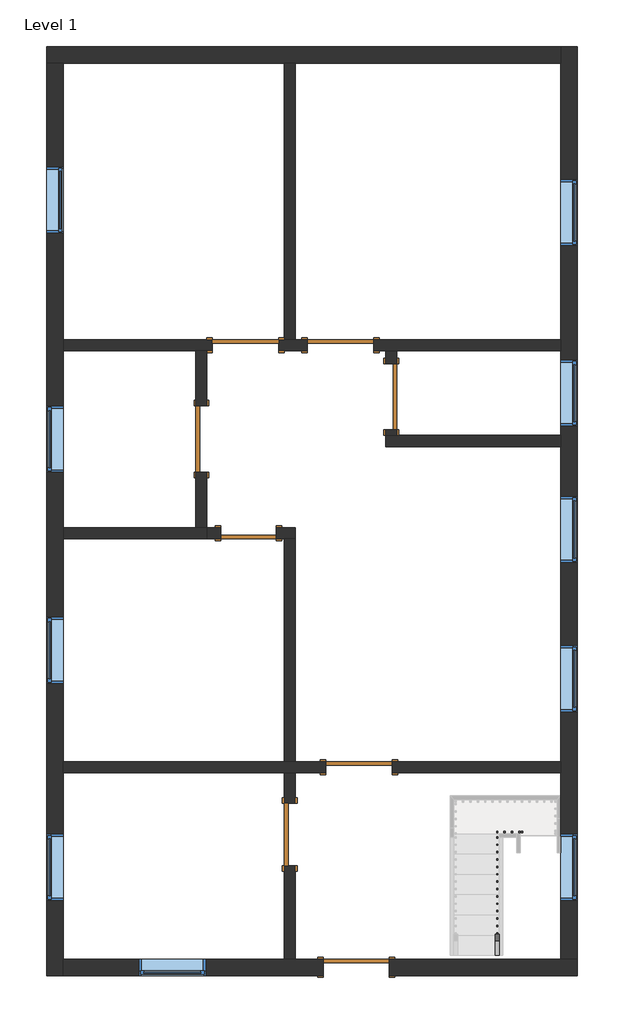
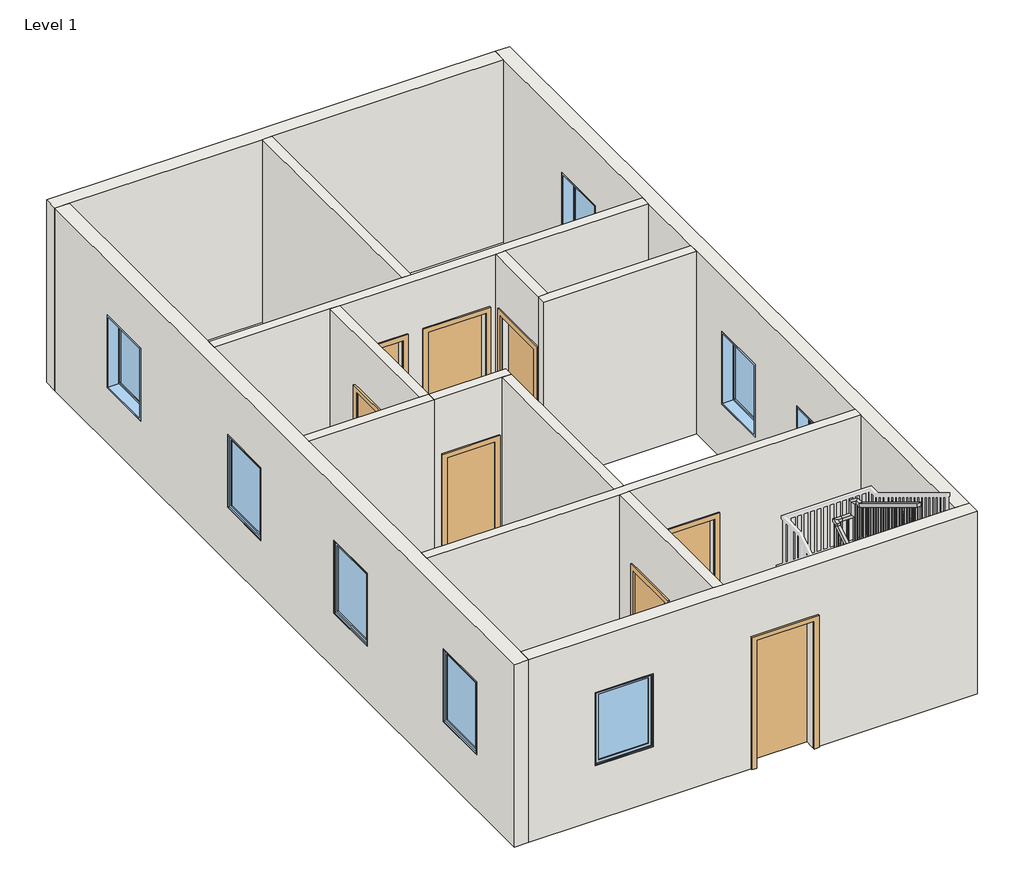
# One storey, part 1 of 2: 13 walls, 10 windows, 8 doors, 1 railing.
"""IFC4 building model written with IfcOpenShell, lengths in millimetres."""

from ifc_helpers import new_model, si_unit, frame, origin, origin_with_axes, place, context, project, spatial, polyline, outline, extrude, faceted_brep, transform, mapped, element, save
from components import door_255cab33, door_56e8e0a9, door_a90ba1ad, door_686f89d2, door_16372e1c, window_c1f32544

model = new_model("IFC4")

# Units and contexts
model_context = context("Model", 3, world=origin())
ifc_project = project(units=[si_unit("LENGTHUNIT", "METRE", prefix="MILLI")], contexts=[model_context])

# Site, building, storey
site = spatial("IfcSite", under=ifc_project)
building = spatial("IfcBuilding", under=site)
storey = spatial("IfcBuildingStorey", under=building, Name="Level 1", Elevation=0.0)

# Doors
placement = place(None, origin())
door_shape = door_255cab33(model_context)
element("IfcDoor", 1, ObjectType="Single-Flush : 30\" x 80\"", at=placement, inside=storey, context=model_context, shape_type="MappedRepresentation", body=[
    mapped(door_shape, transform((-4366.7629117, 1337.2575851, 0.0), x_axis=(1.0, 0.0, 0.0), y_axis=(0.0, 1.0, 0.0), z_axis=(0.0, 0.0, 1.0))),
])
door_2_shape = door_56e8e0a9(model_context)
element("IfcDoor", 2, ObjectType="Single-Flush : 34\" x 80\"", at=placement, inside=storey, context=model_context, shape_type="MappedRepresentation", body=[
    mapped(door_2_shape, transform((-3795.2629117, -2815.6424149, 0.0), x_axis=(0.0, 1.0, 0.0), y_axis=(-1.0, 0.0, 0.0), z_axis=(0.0, 0.0, 1.0))),
])
door_3_shape = door_a90ba1ad(model_context)
element("IfcDoor", 3, ObjectType="Single-Flush : 36\" x 84\"", at=placement, inside=storey, context=model_context, shape_type="MappedRepresentation", body=[
    mapped(door_3_shape, transform((-2880.8629117, -4644.4424149, 0.0), x_axis=(-1.0, 0.0, 0.0), y_axis=(0.0, -1.0, 0.0), z_axis=(0.0, 0.0, 1.0))),
])
door_4_shape = door_686f89d2(model_context)
element("IfcDoor", 4, ObjectType="Single-Flush : 36\" x 84\"", at=placement, inside=storey, context=model_context, shape_type="MappedRepresentation", body=[
    mapped(door_4_shape, transform((-2842.7629117, -1888.5424149, 0.0), x_axis=(-1.0, 0.0, 0.0), y_axis=(0.0, -1.0, 0.0), z_axis=(0.0, 0.0, 1.0))),
])
element("IfcDoor", 5, ObjectType="Single-Flush : 36\" x 84\"", at=placement, inside=storey, context=model_context, shape_type="MappedRepresentation", body=[
    mapped(door_4_shape, transform((-3096.7629117, 3928.0575851, 0.0), x_axis=(-1.0, 0.0, 0.0), y_axis=(0.0, -1.0, 0.0), z_axis=(0.0, 0.0, 1.0))),
])
element("IfcDoor", 6, ObjectType="Single-Flush : 36\" x 84\"", at=placement, inside=storey, context=model_context, shape_type="MappedRepresentation", body=[
    mapped(door_4_shape, transform((-2398.2629117, 3216.8575851, 0.0), x_axis=(0.0, 1.0, 0.0), y_axis=(-1.0, 0.0, 0.0), z_axis=(0.0, 0.0, 1.0))),
])
element("IfcDoor", 7, ObjectType="Single-Flush : 36\" x 84\"", at=placement, inside=storey, context=model_context, shape_type="MappedRepresentation", body=[
    mapped(door_4_shape, transform((-5014.4629117, 2632.6575851, 0.0), x_axis=(0.0, -1.0, 0.0), y_axis=(1.0, 0.0, 0.0), z_axis=(0.0, 0.0, 1.0))),
])
door_5_shape = door_16372e1c(model_context)
element("IfcDoor", 8, ObjectType="Single-Flush : 36\" x 84\"", at=placement, inside=storey, context=model_context, shape_type="MappedRepresentation", body=[
    mapped(door_5_shape, transform((-4404.8629117, 3928.0575851, 0.0), x_axis=(1.0, 0.0, 0.0), y_axis=(0.0, 1.0, 0.0), z_axis=(0.0, 0.0, 1.0))),
])

# Railing
element("IfcRailing", 9, ObjectType="Handrail - Rectangular", at=placement, inside=storey, context=model_context, shape_type="SolidModel", body=[
    faceted_brep([(-963.1629117, -4479.3424149, 1083.7333333), (-963.1629117, -4479.3424149, 1024.3318731), (-912.3629117, -4479.3424149, 1024.3318731), (-912.3629117, -4479.3424149, 1083.7333333), (-963.1629117, -2879.1424149, 2053.5515152), (-963.1629117, -2828.3424149, 2024.9379337), (-912.3629117, -2828.3424149, 2024.9379337), (-912.3629117, -2879.1424149, 2053.5515152), (-963.1629117, -2879.1424149, 2099.7333333), (-963.1629117, -2828.3424149, 2048.9333333), (-912.3629117, -2828.3424149, 2048.9333333), (-912.3629117, -2879.1424149, 2099.7333333), (-963.1629117, -2752.1424149, 2099.7333333), (-963.1629117, -2752.1424149, 2048.9333333), (-912.3629117, -2802.9424149, 2048.9333333), (-912.3629117, -2802.9424149, 2099.7333333), (-836.1629117, -2752.1424149, 2099.7333333), (-836.1629117, -2752.1424149, 2048.9333333), (-836.1629117, -2802.9424149, 2048.9333333), (-836.1629117, -2802.9424149, 2099.7333333), (-696.4629117, -2752.1424149, 2099.7333333), (-645.6629117, -2752.1424149, 2048.9333333), (-645.6629117, -2802.9424149, 2048.9333333), (-696.4629117, -2802.9424149, 2099.7333333), (-696.4629117, -2752.1424149, 2315.2484848), (-645.6629117, -2752.1424149, 2264.4484848), (-645.6629117, -2802.9424149, 2264.4484848), (-696.4629117, -2802.9424149, 2315.2484848), (-569.4629117, -2752.1424149, 2315.2484848), (-569.4629117, -2752.1424149, 2264.4484848), (-620.2629117, -2802.9424149, 2264.4484848), (-620.2629117, -2802.9424149, 2315.2484848), (-569.4629117, -2879.1424149, 2315.2484848), (-569.4629117, -2893.3348244, 2264.4484848), (-620.2629117, -2893.3348244, 2264.4484848), (-620.2629117, -2879.1424149, 2315.2484848), (-569.4629117, -4479.3424149, 3285.0666667), (-620.2629117, -4479.3424149, 3285.0666667), (-620.2629117, -4479.3424149, 3225.6652064), (-569.4629117, -4479.3424149, 3225.6652064)], [[[0, 1, 2, 3]], [[1, 0, 4, 5]], [[2, 1, 5, 6]], [[3, 2, 6, 7]], [[0, 3, 7, 4]], [[5, 4, 8, 9]], [[6, 5, 9, 10]], [[7, 6, 10, 11]], [[4, 7, 11, 8]], [[9, 8, 12, 13]], [[10, 9, 13, 14]], [[11, 10, 14, 15]], [[8, 11, 15, 12]], [[13, 12, 16, 17]], [[14, 13, 17, 18]], [[15, 14, 18, 19]], [[12, 15, 19, 16]], [[17, 16, 20, 21]], [[18, 17, 21, 22]], [[19, 18, 22, 23]], [[16, 19, 23, 20]], [[21, 20, 24, 25]], [[22, 21, 25, 26]], [[23, 22, 26, 27]], [[20, 23, 27, 24]], [[25, 24, 28, 29]], [[26, 25, 29, 30]], [[27, 26, 30, 31]], [[24, 27, 31, 28]], [[29, 28, 32, 33]], [[30, 29, 33, 34]], [[31, 30, 34, 35]], [[28, 31, 35, 32]], [[36, 37, 38, 39]], [[33, 32, 36, 39]], [[34, 33, 39, 38]], [[35, 34, 38, 37]], [[32, 35, 37, 36]]]),
    extrude(outline(polyline([(-4412.6674149, 3185.2561155), (-4393.6174149, 3173.710661), (-4393.6174149, 2201.3333333), (-4412.6674149, 2201.3333333), (-4412.6674149, 3185.2561155)])), frame((-604.3879117, 0.0, 0.0), z_axis=(1.0, 0.0, 0.0), x_axis=(0.0, 1.0, 0.0)), (0.0, 0.0, 1.0), 19.05),
    extrude(outline(polyline([(-4311.0674149, 3123.6803579), (-4292.0174149, 3112.1349034), (-4292.0174149, 2201.3333333), (-4311.0674149, 2201.3333333), (-4311.0674149, 3123.6803579)])), frame((-604.3879117, 0.0, 0.0), z_axis=(1.0, 0.0, 0.0), x_axis=(0.0, 1.0, 0.0)), (0.0, 0.0, 1.0), 19.05),
    extrude(outline(polyline([(-4209.4674149, 3062.1046004), (-4190.4174149, 3050.5591458), (-4190.4174149, 2201.3333333), (-4209.4674149, 2201.3333333), (-4209.4674149, 3062.1046004)])), frame((-604.3879117, 0.0, 0.0), z_axis=(1.0, 0.0, 0.0), x_axis=(0.0, 1.0, 0.0)), (0.0, 0.0, 1.0), 19.05),
    extrude(outline(polyline([(-4107.8674149, 3000.5288428), (-4088.8174149, 2988.9833882), (-4088.8174149, 2032.0), (-4107.8674149, 2032.0), (-4107.8674149, 3000.5288428)])), frame((-604.3879117, 0.0, 0.0), z_axis=(1.0, 0.0, 0.0), x_axis=(0.0, 1.0, 0.0)), (0.0, 0.0, 1.0), 19.05),
    extrude(outline(polyline([(-4006.2674149, 2938.9530852), (-3987.2174149, 2927.4076307), (-3987.2174149, 2032.0), (-4006.2674149, 2032.0), (-4006.2674149, 2938.9530852)])), frame((-604.3879117, 0.0, 0.0), z_axis=(1.0, 0.0, 0.0), x_axis=(0.0, 1.0, 0.0)), (0.0, 0.0, 1.0), 19.05),
    extrude(outline(polyline([(-3904.6674149, 2877.3773276), (-3885.6174149, 2865.8318731), (-3885.6174149, 1862.6666667), (-3904.6674149, 1862.6666667), (-3904.6674149, 2877.3773276)])), frame((-604.3879117, 0.0, 0.0), z_axis=(1.0, 0.0, 0.0), x_axis=(0.0, 1.0, 0.0)), (0.0, 0.0, 1.0), 19.05),
    extrude(outline(polyline([(-3803.0674149, 2815.80157), (-3784.0174149, 2804.2561155), (-3784.0174149, 1862.6666667), (-3803.0674149, 1862.6666667), (-3803.0674149, 2815.80157)])), frame((-604.3879117, 0.0, 0.0), z_axis=(1.0, 0.0, 0.0), x_axis=(0.0, 1.0, 0.0)), (0.0, 0.0, 1.0), 19.05),
    extrude(outline(polyline([(-3701.4674149, 2754.2258125), (-3682.4174149, 2742.6803579), (-3682.4174149, 1862.6666667), (-3701.4674149, 1862.6666667), (-3701.4674149, 2754.2258125)])), frame((-604.3879117, 0.0, 0.0), z_axis=(1.0, 0.0, 0.0), x_axis=(0.0, 1.0, 0.0)), (0.0, 0.0, 1.0), 19.05),
    extrude(outline(polyline([(-3599.8674149, 2692.6500549), (-3580.8174149, 2681.1046004), (-3580.8174149, 1693.3333333), (-3599.8674149, 1693.3333333), (-3599.8674149, 2692.6500549)])), frame((-604.3879117, 0.0, 0.0), z_axis=(1.0, 0.0, 0.0), x_axis=(0.0, 1.0, 0.0)), (0.0, 0.0, 1.0), 19.05),
    extrude(outline(polyline([(-3498.2674149, 2631.0742973), (-3479.2174149, 2619.5288428), (-3479.2174149, 1693.3333333), (-3498.2674149, 1693.3333333), (-3498.2674149, 2631.0742973)])), frame((-604.3879117, 0.0, 0.0), z_axis=(1.0, 0.0, 0.0), x_axis=(0.0, 1.0, 0.0)), (0.0, 0.0, 1.0), 19.05),
    extrude(outline(polyline([(-3396.6674149, 2569.4985397), (-3377.6174149, 2557.9530852), (-3377.6174149, 1693.3333333), (-3396.6674149, 1693.3333333), (-3396.6674149, 2569.4985397)])), frame((-604.3879117, 0.0, 0.0), z_axis=(1.0, 0.0, 0.0), x_axis=(0.0, 1.0, 0.0)), (0.0, 0.0, 1.0), 19.05),
    extrude(outline(polyline([(-3295.0674149, 2507.9227822), (-3276.0174149, 2496.3773276), (-3276.0174149, 1524.0), (-3295.0674149, 1524.0), (-3295.0674149, 2507.9227822)])), frame((-604.3879117, 0.0, 0.0), z_axis=(1.0, 0.0, 0.0), x_axis=(0.0, 1.0, 0.0)), (0.0, 0.0, 1.0), 19.05),
    extrude(outline(polyline([(-3193.4674149, 2446.3470246), (-3174.4174149, 2434.80157), (-3174.4174149, 1524.0), (-3193.4674149, 1524.0), (-3193.4674149, 2446.3470246)])), frame((-604.3879117, 0.0, 0.0), z_axis=(1.0, 0.0, 0.0), x_axis=(0.0, 1.0, 0.0)), (0.0, 0.0, 1.0), 19.05),
    extrude(outline(polyline([(-3091.8674149, 2384.771267), (-3072.8174149, 2373.2258125), (-3072.8174149, 1524.0), (-3091.8674149, 1524.0), (-3091.8674149, 2384.771267)])), frame((-604.3879117, 0.0, 0.0), z_axis=(1.0, 0.0, 0.0), x_axis=(0.0, 1.0, 0.0)), (0.0, 0.0, 1.0), 19.05),
    extrude(outline(polyline([(-2990.2674149, 2323.1955094), (-2971.2174149, 2311.6500549), (-2971.2174149, 1354.6666667), (-2990.2674149, 1354.6666667), (-2990.2674149, 2323.1955094)])), frame((-604.3879117, 0.0, 0.0), z_axis=(1.0, 0.0, 0.0), x_axis=(0.0, 1.0, 0.0)), (0.0, 0.0, 1.0), 19.05),
    extrude(outline(polyline([(-2888.6674149, 2261.6197519), (-2869.6174149, 2250.0742973), (-2869.6174149, 1354.6666667), (-2888.6674149, 1354.6666667), (-2888.6674149, 2261.6197519)])), frame((-604.3879117, 0.0, 0.0), z_axis=(1.0, 0.0, 0.0), x_axis=(0.0, 1.0, 0.0)), (0.0, 0.0, 1.0), 19.05),
    extrude(outline(polyline([(-642.4879117, -2787.0674149), (-642.4879117, -2768.0174149), (-623.4379117, -2768.0174149), (-623.4379117, -2787.0674149), (-642.4879117, -2787.0674149)])), frame((0.0, 0.0, 1185.3333333), z_axis=(0.0, 0.0, 1.0), x_axis=(1.0, 0.0, 0.0)), (0.0, 0.0, 1.0), 1079.1151515),
    extrude(outline(polyline([(-744.0879117, -2787.0674149), (-744.0879117, -2768.0174149), (-725.0379117, -2768.0174149), (-725.0379117, -2787.0674149), (-744.0879117, -2787.0674149)])), frame((0.0, 0.0, 1185.3333333), z_axis=(0.0, 0.0, 1.0), x_axis=(1.0, 0.0, 0.0)), (0.0, 0.0, 1.0), 863.6),
    extrude(outline(polyline([(-845.6879117, -2787.0674149), (-845.6879117, -2768.0174149), (-826.6379117, -2768.0174149), (-826.6379117, -2787.0674149), (-845.6879117, -2787.0674149)])), frame((0.0, 0.0, 1185.3333333), z_axis=(0.0, 0.0, 1.0), x_axis=(1.0, 0.0, 0.0)), (0.0, 0.0, 1.0), 863.6),
    extrude(outline(polyline([(-928.2379117, -2863.2674149), (-947.2879117, -2863.2674149), (-947.2879117, -2844.2174149), (-928.2379117, -2844.2174149), (-928.2379117, -2863.2674149)])), frame((0.0, 0.0, 1016.0), z_axis=(0.0, 0.0, 1.0), x_axis=(1.0, 0.0, 0.0)), (0.0, 0.0, 1.0), 1032.9333333),
    extrude(outline(polyline([(-2964.8674149, 1942.1955094), (-2945.8174149, 1953.740964), (-2945.8174149, 1016.0), (-2964.8674149, 1016.0), (-2964.8674149, 1942.1955094)])), frame((-947.2879117, 0.0, 0.0), z_axis=(1.0, 0.0, 0.0), x_axis=(0.0, 1.0, 0.0)), (0.0, 0.0, 1.0), 19.05),
    extrude(outline(polyline([(-3066.4674149, 1880.6197519), (-3047.4174149, 1892.1652064), (-3047.4174149, 1016.0), (-3066.4674149, 1016.0), (-3066.4674149, 1880.6197519)])), frame((-947.2879117, 0.0, 0.0), z_axis=(1.0, 0.0, 0.0), x_axis=(0.0, 1.0, 0.0)), (0.0, 0.0, 1.0), 19.05),
    extrude(outline(polyline([(-3168.0674149, 1819.0439943), (-3149.0174149, 1830.5894488), (-3149.0174149, 846.6666667), (-3168.0674149, 846.6666667), (-3168.0674149, 1819.0439943)])), frame((-947.2879117, 0.0, 0.0), z_axis=(1.0, 0.0, 0.0), x_axis=(0.0, 1.0, 0.0)), (0.0, 0.0, 1.0), 19.05),
    extrude(outline(polyline([(-3269.6674149, 1757.4682367), (-3250.6174149, 1769.0136913), (-3250.6174149, 846.6666667), (-3269.6674149, 846.6666667), (-3269.6674149, 1757.4682367)])), frame((-947.2879117, 0.0, 0.0), z_axis=(1.0, 0.0, 0.0), x_axis=(0.0, 1.0, 0.0)), (0.0, 0.0, 1.0), 19.05),
    extrude(outline(polyline([(-3371.2674149, 1695.8924791), (-3352.2174149, 1707.4379337), (-3352.2174149, 846.6666667), (-3371.2674149, 846.6666667), (-3371.2674149, 1695.8924791)])), frame((-947.2879117, 0.0, 0.0), z_axis=(1.0, 0.0, 0.0), x_axis=(0.0, 1.0, 0.0)), (0.0, 0.0, 1.0), 19.05),
    extrude(outline(polyline([(-3472.8674149, 1634.3167216), (-3453.8174149, 1645.8621761), (-3453.8174149, 677.3333333), (-3472.8674149, 677.3333333), (-3472.8674149, 1634.3167216)])), frame((-947.2879117, 0.0, 0.0), z_axis=(1.0, 0.0, 0.0), x_axis=(0.0, 1.0, 0.0)), (0.0, 0.0, 1.0), 19.05),
    extrude(outline(polyline([(-3574.4674149, 1572.740964), (-3555.4174149, 1584.2864185), (-3555.4174149, 677.3333333), (-3574.4674149, 677.3333333), (-3574.4674149, 1572.740964)])), frame((-947.2879117, 0.0, 0.0), z_axis=(1.0, 0.0, 0.0), x_axis=(0.0, 1.0, 0.0)), (0.0, 0.0, 1.0), 19.05),
    extrude(outline(polyline([(-3676.0674149, 1511.1652064), (-3657.0174149, 1522.710661), (-3657.0174149, 508.0), (-3676.0674149, 508.0), (-3676.0674149, 1511.1652064)])), frame((-947.2879117, 0.0, 0.0), z_axis=(1.0, 0.0, 0.0), x_axis=(0.0, 1.0, 0.0)), (0.0, 0.0, 1.0), 19.05),
    extrude(outline(polyline([(-3777.6674149, 1449.5894488), (-3758.6174149, 1461.1349034), (-3758.6174149, 508.0), (-3777.6674149, 508.0), (-3777.6674149, 1449.5894488)])), frame((-947.2879117, 0.0, 0.0), z_axis=(1.0, 0.0, 0.0), x_axis=(0.0, 1.0, 0.0)), (0.0, 0.0, 1.0), 19.05),
    extrude(outline(polyline([(-3879.2674149, 1388.0136913), (-3860.2174149, 1399.5591458), (-3860.2174149, 508.0), (-3879.2674149, 508.0), (-3879.2674149, 1388.0136913)])), frame((-947.2879117, 0.0, 0.0), z_axis=(1.0, 0.0, 0.0), x_axis=(0.0, 1.0, 0.0)), (0.0, 0.0, 1.0), 19.05),
    extrude(outline(polyline([(-3980.8674149, 1326.4379337), (-3961.8174149, 1337.9833882), (-3961.8174149, 338.6666667), (-3980.8674149, 338.6666667), (-3980.8674149, 1326.4379337)])), frame((-947.2879117, 0.0, 0.0), z_axis=(1.0, 0.0, 0.0), x_axis=(0.0, 1.0, 0.0)), (0.0, 0.0, 1.0), 19.05),
    extrude(outline(polyline([(-4082.4674149, 1264.8621761), (-4063.4174149, 1276.4076307), (-4063.4174149, 338.6666667), (-4082.4674149, 338.6666667), (-4082.4674149, 1264.8621761)])), frame((-947.2879117, 0.0, 0.0), z_axis=(1.0, 0.0, 0.0), x_axis=(0.0, 1.0, 0.0)), (0.0, 0.0, 1.0), 19.05),
    extrude(outline(polyline([(-4184.0674149, 1203.2864185), (-4165.0174149, 1214.8318731), (-4165.0174149, 338.6666667), (-4184.0674149, 338.6666667), (-4184.0674149, 1203.2864185)])), frame((-947.2879117, 0.0, 0.0), z_axis=(1.0, 0.0, 0.0), x_axis=(0.0, 1.0, 0.0)), (0.0, 0.0, 1.0), 19.05),
    extrude(outline(polyline([(-4285.6674149, 1141.710661), (-4266.6174149, 1153.2561155), (-4266.6174149, 169.3333333), (-4285.6674149, 169.3333333), (-4285.6674149, 1141.710661)])), frame((-947.2879117, 0.0, 0.0), z_axis=(1.0, 0.0, 0.0), x_axis=(0.0, 1.0, 0.0)), (0.0, 0.0, 1.0), 19.05),
    extrude(outline(polyline([(-4387.2674149, 1080.1349034), (-4368.2174149, 1091.6803579), (-4368.2174149, 169.3333333), (-4387.2674149, 169.3333333), (-4387.2674149, 1080.1349034)])), frame((-947.2879117, 0.0, 0.0), z_axis=(1.0, 0.0, 0.0), x_axis=(0.0, 1.0, 0.0)), (0.0, 0.0, 1.0), 19.05),
    extrude(outline(polyline([(-604.3879117, -2787.0674149), (-604.3879117, -2768.0174149), (-585.3379117, -2768.0174149), (-585.3379117, -2787.0674149), (-604.3879117, -2787.0674149)])), frame((0.0, 0.0, 1185.3333333), z_axis=(0.0, 0.0, 1.0), x_axis=(1.0, 0.0, 0.0)), (0.0, 0.0, 1.0), 1079.1151515),
    extrude(outline(polyline([(-928.2379117, -2787.0674149), (-947.2879117, -2787.0674149), (-947.2879117, -2768.0174149), (-928.2379117, -2768.0174149), (-928.2379117, -2787.0674149)])), frame((0.0, 0.0, 1185.3333333), z_axis=(0.0, 0.0, 1.0), x_axis=(1.0, 0.0, 0.0)), (0.0, 0.0, 1.0), 863.6),
    extrude(outline(polyline([(-4479.3424149, 3225.6652064), (-4460.2924149, 3214.1197519), (-4460.2924149, 2201.3333333), (-4479.3424149, 2201.3333333), (-4479.3424149, 3225.6652064)])), frame((-604.3879117, 0.0, 0.0), z_axis=(1.0, 0.0, 0.0), x_axis=(0.0, 1.0, 0.0)), (0.0, 0.0, 1.0), 19.05),
    extrude(outline(polyline([(-4479.3424149, 1024.3318731), (-4460.2924149, 1035.8773276), (-4460.2924149, 169.3333333), (-4479.3424149, 169.3333333), (-4479.3424149, 1024.3318731)])), frame((-947.2879117, 0.0, 0.0), z_axis=(1.0, 0.0, 0.0), x_axis=(0.0, 1.0, 0.0)), (0.0, 0.0, 1.0), 19.05),
])

# Walls
element("IfcWall", 10, ObjectType="Generic - 6\"", at=placement, inside=storey, context=model_context, shape_type="SweptSolid", body=[
    extrude(outline(polyline([(-3719.0629117, 7814.2575851), (-3719.0629117, 4004.2575851), (-3871.4629117, 4004.2575851), (-3871.4629117, 7814.2575851), (-3719.0629117, 7814.2575851)])), origin_with_axes(), (0.0, 0.0, 1.0), 3048.0),
])
element("IfcWall", 11, ObjectType="Generic - 6\"", at=placement, inside=storey, context=model_context, shape_type="Brep", body=[
    faceted_brep([(-3947.6629117, 3851.8575851, 2133.6), (-3947.6629117, 3851.8575851, 0.0), (-3553.9629117, 3851.8575851, 0.0), (-3553.9629117, 3851.8575851, 2133.6), (-2639.5629117, 3851.8575851, 2133.6), (-2639.5629117, 3851.8575851, 0.0), (-2474.4629117, 3851.8575851, 0.0), (-2322.0629117, 3851.8575851, 0.0), (-61.4629117, 3851.8575851, 0.0), (-61.4629117, 3851.8575851, 3048.0), (-2322.0629117, 3851.8575851, 3048.0), (-2474.4629117, 3851.8575851, 3048.0), (-4938.2629117, 3851.8575851, 3048.0), (-5090.6629117, 3851.8575851, 3048.0), (-6919.4629117, 3851.8575851, 3048.0), (-6919.4629117, 3851.8575851, 0.0), (-5090.6629117, 3851.8575851, 0.0), (-4938.2629117, 3851.8575851, 0.0), (-4862.0629117, 3851.8575851, 0.0), (-4862.0629117, 3851.8575851, 2133.6), (-3553.9629117, 4004.2575851, 0.0), (-3719.0629117, 4004.2575851, 0.0), (-3871.4629117, 4004.2575851, 0.0), (-3947.6629117, 4004.2575851, 0.0), (-3947.6629117, 4004.2575851, 2133.6), (-4862.0629117, 4004.2575851, 2133.6), (-4862.0629117, 4004.2575851, 0.0), (-6919.4629117, 4004.2575851, 0.0), (-6919.4629117, 4004.2575851, 3048.0), (-3871.4629117, 4004.2575851, 3048.0), (-3719.0629117, 4004.2575851, 3048.0), (-61.4629117, 4004.2575851, 3048.0), (-61.4629117, 4004.2575851, 0.0), (-2639.5629117, 4004.2575851, 0.0), (-2639.5629117, 4004.2575851, 2133.6), (-3553.9629117, 4004.2575851, 2133.6)], [[[0, 1, 2, 3, 4, 5, 6, 7, 8, 9, 10, 11, 12, 13, 14, 15, 16, 17, 18, 19]], [[20, 21, 22, 23, 24, 25, 26, 27, 28, 29, 30, 31, 32, 33, 34, 35]], [[33, 32, 8, 7, 6, 5]], [[2, 1, 23, 22, 21, 20]], [[18, 17, 16, 15, 27, 26]], [[14, 13, 12, 11, 10, 9, 31, 30, 29, 28]], [[15, 14, 28, 27]], [[9, 8, 32, 31]], [[3, 2, 20, 35]], [[4, 3, 35, 34]], [[5, 4, 34, 33]], [[24, 23, 1, 0]], [[25, 24, 0, 19]], [[26, 25, 19, 18]]]),
])
element("IfcWall", 12, ObjectType="Generic - 6\"", at=placement, inside=storey, context=model_context, shape_type="Brep", body=[
    faceted_brep([(-2474.4629117, 2531.0575851, 0.0), (-61.4629117, 2531.0575851, 0.0), (-61.4629117, 2531.0575851, 3048.0), (-2474.4629117, 2531.0575851, 3048.0), (-2474.4629117, 2683.4575851, 0.0), (-2474.4629117, 2683.4575851, 3048.0), (-2322.0629117, 2683.4575851, 3048.0), (-61.4629117, 2683.4575851, 3048.0), (-61.4629117, 2683.4575851, 0.0), (-2322.0629117, 2683.4575851, 0.0)], [[[0, 1, 2, 3]], [[4, 5, 6, 7, 8, 9]], [[1, 0, 4, 9, 8]], [[3, 2, 7, 6, 5]], [[2, 1, 8, 7]], [[0, 3, 5, 4]]]),
])
element("IfcWall", 13, ObjectType="Generic - 6\"", at=placement, inside=storey, context=model_context, shape_type="SweptSolid", body=[
    extrude(outline(polyline([(3851.8575851, 0.0), (3674.0575851, 0.0), (3674.0575851, 2133.6), (2759.6575851, 2133.6), (2759.6575851, 0.0), (2683.4575851, 0.0), (2683.4575851, 3048.0), (3851.8575851, 3048.0), (3851.8575851, 0.0)])), frame((-2474.4629117, 0.0, 0.0), z_axis=(1.0, 0.0, 0.0), x_axis=(0.0, 1.0, 0.0)), (0.0, 0.0, 1.0), 152.4),
])
element("IfcWall", 14, ObjectType="Generic - 6\"", at=placement, inside=storey, context=model_context, shape_type="Brep", body=[
    faceted_brep([(-6919.4629117, 1261.0575851, 0.0), (-4938.2629117, 1261.0575851, 0.0), (-4938.2629117, 1261.0575851, 3048.0), (-6919.4629117, 1261.0575851, 3048.0), (-6919.4629117, 1413.4575851, 0.0), (-6919.4629117, 1413.4575851, 3048.0), (-5090.6629117, 1413.4575851, 3048.0), (-4938.2629117, 1413.4575851, 3048.0), (-4938.2629117, 1413.4575851, 0.0), (-5090.6629117, 1413.4575851, 0.0)], [[[0, 1, 2, 3]], [[4, 5, 6, 7, 8, 9]], [[1, 0, 4, 9, 8]], [[3, 2, 7, 6, 5]], [[0, 3, 5, 4]], [[2, 1, 8, 7]]]),
])
element("IfcWall", 15, ObjectType="Generic - 6\"", at=placement, inside=storey, context=model_context, shape_type="SweptSolid", body=[
    extrude(outline(polyline([(2175.4575851, 2133.6), (2175.4575851, 0.0), (1413.4575851, 0.0), (1413.4575851, 3048.0), (3851.8575851, 3048.0), (3851.8575851, 0.0), (3089.8575851, 0.0), (3089.8575851, 2133.6), (2175.4575851, 2133.6)])), frame((-5090.6629117, 0.0, 0.0), z_axis=(1.0, 0.0, 0.0), x_axis=(0.0, 1.0, 0.0)), (0.0, 0.0, 1.0), 152.4),
])
element("IfcWall", 16, ObjectType="Generic - 6\"", at=placement, inside=storey, context=model_context, shape_type="Brep", body=[
    faceted_brep([(-6919.4629117, -1964.7424149, 0.0), (-3871.4629117, -1964.7424149, 0.0), (-3719.0629117, -1964.7424149, 0.0), (-3299.9629117, -1964.7424149, 0.0), (-3299.9629117, -1964.7424149, 2133.6), (-2385.5629117, -1964.7424149, 2133.6), (-2385.5629117, -1964.7424149, 0.0), (-61.4629117, -1964.7424149, 0.0), (-61.4629117, -1964.7424149, 3048.0), (-3719.0629117, -1964.7424149, 3048.0), (-3871.4629117, -1964.7424149, 3048.0), (-6919.4629117, -1964.7424149, 3048.0), (-3299.9629117, -1812.3424149, 2133.6), (-3299.9629117, -1812.3424149, 0.0), (-3719.0629117, -1812.3424149, 0.0), (-3871.4629117, -1812.3424149, 0.0), (-6919.4629117, -1812.3424149, 0.0), (-6919.4629117, -1812.3424149, 3048.0), (-3871.4629117, -1812.3424149, 3048.0), (-3719.0629117, -1812.3424149, 3048.0), (-61.4629117, -1812.3424149, 3048.0), (-61.4629117, -1812.3424149, 0.0), (-2385.5629117, -1812.3424149, 0.0), (-2385.5629117, -1812.3424149, 2133.6)], [[[0, 1, 2, 3, 4, 5, 6, 7, 8, 9, 10, 11]], [[12, 13, 14, 15, 16, 17, 18, 19, 20, 21, 22, 23]], [[22, 21, 7, 6]], [[16, 15, 14, 13, 3, 2, 1, 0]], [[11, 10, 9, 8, 20, 19, 18, 17]], [[0, 11, 17, 16]], [[8, 7, 21, 20]], [[4, 3, 13, 12]], [[5, 4, 12, 23]], [[6, 5, 23, 22]]]),
])
element("IfcWall", 17, ObjectType="Generic - 6\"", at=placement, inside=storey, context=model_context, shape_type="SweptSolid", body=[
    extrude(outline(polyline([(-4530.1424149, 0.0), (-4530.1424149, 3048.0), (-1964.7424149, 3048.0), (-1964.7424149, 0.0), (-2383.8424149, 0.0), (-2383.8424149, 2032.0), (-3247.4424149, 2032.0), (-3247.4424149, 0.0), (-4530.1424149, 0.0)])), frame((-3871.4629117, 0.0, 0.0), z_axis=(1.0, 0.0, 0.0), x_axis=(0.0, 1.0, 0.0)), (0.0, 0.0, 1.0), 152.4),
    extrude(outline(polyline([(-3871.4629117, 1261.0575851), (-3719.0629117, 1261.0575851), (-3719.0629117, -1812.3424149), (-3871.4629117, -1812.3424149), (-3871.4629117, 1261.0575851)])), origin_with_axes(), (0.0, 0.0, 1.0), 3048.0),
])
element("IfcWall", 18, ObjectType="Generic - 6\"", at=placement, inside=storey, context=model_context, shape_type="Brep", body=[
    faceted_brep([(-3985.7629117, 1261.0575851, 2032.0), (-3985.7629117, 1261.0575851, 0.0), (-3871.4629117, 1261.0575851, 0.0), (-3719.0629117, 1261.0575851, 0.0), (-3719.0629117, 1261.0575851, 3048.0), (-3871.4629117, 1261.0575851, 3048.0), (-4938.2629117, 1261.0575851, 3048.0), (-4938.2629117, 1261.0575851, 0.0), (-4747.7629117, 1261.0575851, 0.0), (-4747.7629117, 1261.0575851, 2032.0), (-3719.0629117, 1413.4575851, 0.0), (-3985.7629117, 1413.4575851, 0.0), (-3985.7629117, 1413.4575851, 2032.0), (-4747.7629117, 1413.4575851, 2032.0), (-4747.7629117, 1413.4575851, 0.0), (-4938.2629117, 1413.4575851, 0.0), (-4938.2629117, 1413.4575851, 3048.0), (-3719.0629117, 1413.4575851, 3048.0)], [[[0, 1, 2, 3, 4, 5, 6, 7, 8, 9]], [[10, 11, 12, 13, 14, 15, 16, 17]], [[8, 7, 15, 14]], [[3, 2, 1, 11, 10]], [[4, 3, 10, 17]], [[6, 5, 4, 17, 16]], [[7, 6, 16, 15]], [[12, 11, 1, 0]], [[13, 12, 0, 9]], [[14, 13, 9, 8]]]),
])
element("IfcWall", 19, ObjectType="Generic - 9\"", at=placement, inside=storey, context=model_context, shape_type="Brep", body=[
    faceted_brep([(-7148.0629117, 7814.2575851, 0.0), (-6919.4629117, 7814.2575851, 0.0), (-3871.4629117, 7814.2575851, 0.0), (-3719.0629117, 7814.2575851, 0.0), (-61.4629117, 7814.2575851, 0.0), (-61.4629117, 7814.2575851, 3048.0), (-3719.0629117, 7814.2575851, 3048.0), (-3871.4629117, 7814.2575851, 3048.0), (-6919.4629117, 7814.2575851, 3048.0), (-7148.0629117, 7814.2575851, 3048.0), (-7148.0629117, 8042.8575851, 0.0), (-7148.0629117, 8042.8575851, 3048.0), (-61.4629117, 8042.8575851, 3048.0), (-61.4629117, 8042.8575851, 0.0)], [[[0, 1, 2, 3, 4, 5, 6, 7, 8, 9]], [[10, 11, 12, 13]], [[4, 3, 2, 1, 0, 10, 13]], [[9, 8, 7, 6, 5, 12, 11]], [[0, 9, 11, 10]], [[5, 4, 13, 12]]]),
])
element("IfcWall", 20, ObjectType="Generic - 9\"", at=placement, inside=storey, context=model_context, shape_type="Brep", body=[
    faceted_brep([(-6919.4629117, -4758.7424149, 0.0), (-6919.4629117, -4530.1424149, 0.0), (-6919.4629117, -1964.7424149, 0.0), (-6919.4629117, -1812.3424149, 0.0), (-6919.4629117, 1261.0575851, 0.0), (-6919.4629117, 1413.4575851, 0.0), (-6919.4629117, 3851.8575851, 0.0), (-6919.4629117, 4004.2575851, 0.0), (-6919.4629117, 7814.2575851, 0.0), (-6919.4629117, 7814.2575851, 3048.0), (-6919.4629117, 4004.2575851, 3048.0), (-6919.4629117, 3851.8575851, 3048.0), (-6919.4629117, 1413.4575851, 3048.0), (-6919.4629117, 1261.0575851, 3048.0), (-6919.4629117, -1812.3424149, 3048.0), (-6919.4629117, -1964.7424149, 3048.0), (-6919.4629117, -4530.1424149, 3048.0), (-6919.4629117, -4758.7424149, 3048.0), (-6919.4629117, 5471.1075851, 2133.6), (-6919.4629117, 6385.5075851, 2133.6), (-6919.4629117, 6385.5075851, 914.4), (-6919.4629117, 5471.1075851, 914.4), (-6919.4629117, 3089.8575851, 2133.6), (-6919.4629117, 3089.8575851, 914.4), (-6919.4629117, 2175.4575851, 914.4), (-6919.4629117, 2175.4575851, 2133.6), (-6919.4629117, 181.5575851, 2133.6), (-6919.4629117, 181.5575851, 914.4), (-6919.4629117, -732.8424149, 914.4), (-6919.4629117, -732.8424149, 2133.6), (-6919.4629117, -2809.2924149, 2133.6), (-6919.4629117, -2809.2924149, 914.4), (-6919.4629117, -3723.6924149, 914.4), (-6919.4629117, -3723.6924149, 2133.6), (-7148.0629117, -4758.7424149, 0.0), (-7148.0629117, -4758.7424149, 3048.0), (-7148.0629117, 7814.2575851, 3048.0), (-7148.0629117, 7814.2575851, 0.0), (-7148.0629117, 5471.1075851, 2133.6), (-7148.0629117, 5471.1075851, 914.4), (-7148.0629117, 6385.5075851, 914.4), (-7148.0629117, 6385.5075851, 2133.6), (-7148.0629117, 3089.8575851, 2133.6), (-7148.0629117, 2175.4575851, 2133.6), (-7148.0629117, 2175.4575851, 914.4), (-7148.0629117, 3089.8575851, 914.4), (-7148.0629117, 181.5575851, 2133.6), (-7148.0629117, -732.8424149, 2133.6), (-7148.0629117, -732.8424149, 914.4), (-7148.0629117, 181.5575851, 914.4), (-7148.0629117, -2809.2924149, 2133.6), (-7148.0629117, -3723.6924149, 2133.6), (-7148.0629117, -3723.6924149, 914.4), (-7148.0629117, -2809.2924149, 914.4)], [[[0, 1, 2, 3, 4, 5, 6, 7, 8, 9, 10, 11, 12, 13, 14, 15, 16, 17], [18, 19, 20, 21], [22, 23, 24, 25], [26, 27, 28, 29], [30, 31, 32, 33]], [[34, 35, 36, 37], [38, 39, 40, 41], [42, 43, 44, 45], [46, 47, 48, 49], [50, 51, 52, 53]], [[8, 7, 6, 5, 4, 3, 2, 1, 0, 34, 37]], [[17, 16, 15, 14, 13, 12, 11, 10, 9, 36, 35]], [[0, 17, 35, 34]], [[9, 8, 37, 36]], [[39, 38, 18, 21]], [[40, 39, 21, 20]], [[41, 40, 20, 19]], [[38, 41, 19, 18]], [[23, 22, 42, 45]], [[24, 23, 45, 44]], [[25, 24, 44, 43]], [[22, 25, 43, 42]], [[27, 26, 46, 49]], [[28, 27, 49, 48]], [[29, 28, 48, 47]], [[26, 29, 47, 46]], [[31, 30, 50, 53]], [[32, 31, 53, 52]], [[33, 32, 52, 51]], [[30, 33, 51, 50]]]),
])
element("IfcWall", 21, ObjectType="Generic - 9\"", at=placement, inside=storey, context=model_context, shape_type="Brep", body=[
    faceted_brep([(-3338.0629117, -4530.1424149, 2133.6), (-3338.0629117, -4530.1424149, 0.0), (-3719.0629117, -4530.1424149, 0.0), (-3871.4629117, -4530.1424149, 0.0), (-6919.4629117, -4530.1424149, 0.0), (-6919.4629117, -4530.1424149, 3048.0), (-3871.4629117, -4530.1424149, 3048.0), (-3719.0629117, -4530.1424149, 3048.0), (-61.4629117, -4530.1424149, 3048.0), (167.1370883, -4530.1424149, 3048.0), (167.1370883, -4530.1424149, 0.0), (-61.4629117, -4530.1424149, 0.0), (-2423.6629117, -4530.1424149, 0.0), (-2423.6629117, -4530.1424149, 2133.6), (-5871.7129117, -4530.1424149, 2133.6), (-5871.7129117, -4530.1424149, 914.4), (-4957.3129117, -4530.1424149, 914.4), (-4957.3129117, -4530.1424149, 2133.6), (-6919.4629117, -4758.7424149, 0.0), (-3338.0629117, -4758.7424149, 0.0), (-3338.0629117, -4758.7424149, 2133.6), (-2423.6629117, -4758.7424149, 2133.6), (-2423.6629117, -4758.7424149, 0.0), (167.1370883, -4758.7424149, 0.0), (167.1370883, -4758.7424149, 3048.0), (-6919.4629117, -4758.7424149, 3048.0), (-5871.7129117, -4758.7424149, 2133.6), (-4957.3129117, -4758.7424149, 2133.6), (-4957.3129117, -4758.7424149, 914.4), (-5871.7129117, -4758.7424149, 914.4)], [[[0, 1, 2, 3, 4, 5, 6, 7, 8, 9, 10, 11, 12, 13], [14, 15, 16, 17]], [[18, 19, 20, 21, 22, 23, 24, 25], [26, 27, 28, 29]], [[12, 11, 10, 23, 22]], [[4, 3, 2, 1, 19, 18]], [[9, 8, 7, 6, 5, 25, 24]], [[10, 9, 24, 23]], [[5, 4, 18, 25]], [[20, 19, 1, 0]], [[21, 20, 0, 13]], [[22, 21, 13, 12]], [[15, 14, 26, 29]], [[16, 15, 29, 28]], [[17, 16, 28, 27]], [[14, 17, 27, 26]]]),
])
element("IfcWall", 22, ObjectType="Generic - 9\"", at=placement, inside=storey, context=model_context, shape_type="Brep", body=[
    faceted_brep([(-61.4629117, 8042.8575851, 0.0), (-61.4629117, 7814.2575851, 0.0), (-61.4629117, 4004.2575851, 0.0), (-61.4629117, 3851.8575851, 0.0), (-61.4629117, 2683.4575851, 0.0), (-61.4629117, 2531.0575851, 0.0), (-61.4629117, -1812.3424149, 0.0), (-61.4629117, -1964.7424149, 0.0), (-61.4629117, -4530.1424149, 0.0), (-61.4629117, -4530.1424149, 3048.0), (-61.4629117, -1964.7424149, 3048.0), (-61.4629117, -1812.3424149, 3048.0), (-61.4629117, 2531.0575851, 3048.0), (-61.4629117, 2683.4575851, 3048.0), (-61.4629117, 3851.8575851, 3048.0), (-61.4629117, 4004.2575851, 3048.0), (-61.4629117, 7814.2575851, 3048.0), (-61.4629117, 8042.8575851, 3048.0), (-61.4629117, -3723.6924149, 2133.6), (-61.4629117, -3723.6924149, 914.4), (-61.4629117, -2809.2924149, 914.4), (-61.4629117, -2809.2924149, 2133.6), (-61.4629117, -1126.5424149, 2133.6), (-61.4629117, -1126.5424149, 914.4), (-61.4629117, -212.1424149, 914.4), (-61.4629117, -212.1424149, 2133.6), (-61.4629117, 930.8575851, 2133.6), (-61.4629117, 930.8575851, 914.4), (-61.4629117, 1845.2575851, 914.4), (-61.4629117, 1845.2575851, 2133.6), (-61.4629117, 2810.4575851, 2133.6), (-61.4629117, 2810.4575851, 914.4), (-61.4629117, 3724.8575851, 914.4), (-61.4629117, 3724.8575851, 2133.6), (-61.4629117, 5299.6575851, 2133.6), (-61.4629117, 5299.6575851, 914.4), (-61.4629117, 6214.0575851, 914.4), (-61.4629117, 6214.0575851, 2133.6), (167.1370883, 8042.8575851, 0.0), (167.1370883, 8042.8575851, 3048.0), (167.1370883, -4530.1424149, 3048.0), (167.1370883, -4530.1424149, 0.0), (167.1370883, -3723.6924149, 2133.6), (167.1370883, -2809.2924149, 2133.6), (167.1370883, -2809.2924149, 914.4), (167.1370883, -3723.6924149, 914.4), (167.1370883, -1126.5424149, 2133.6), (167.1370883, -212.1424149, 2133.6), (167.1370883, -212.1424149, 914.4), (167.1370883, -1126.5424149, 914.4), (167.1370883, 930.8575851, 2133.6), (167.1370883, 1845.2575851, 2133.6), (167.1370883, 1845.2575851, 914.4), (167.1370883, 930.8575851, 914.4), (167.1370883, 2810.4575851, 2133.6), (167.1370883, 3724.8575851, 2133.6), (167.1370883, 3724.8575851, 914.4), (167.1370883, 2810.4575851, 914.4), (167.1370883, 5299.6575851, 2133.6), (167.1370883, 6214.0575851, 2133.6), (167.1370883, 6214.0575851, 914.4), (167.1370883, 5299.6575851, 914.4)], [[[0, 1, 2, 3, 4, 5, 6, 7, 8, 9, 10, 11, 12, 13, 14, 15, 16, 17], [18, 19, 20, 21], [22, 23, 24, 25], [26, 27, 28, 29], [30, 31, 32, 33], [34, 35, 36, 37]], [[38, 39, 40, 41], [42, 43, 44, 45], [46, 47, 48, 49], [50, 51, 52, 53], [54, 55, 56, 57], [58, 59, 60, 61]], [[8, 7, 6, 5, 4, 3, 2, 1, 0, 38, 41]], [[17, 16, 15, 14, 13, 12, 11, 10, 9, 40, 39]], [[0, 17, 39, 38]], [[9, 8, 41, 40]], [[19, 18, 42, 45]], [[20, 19, 45, 44]], [[21, 20, 44, 43]], [[18, 21, 43, 42]], [[23, 22, 46, 49]], [[24, 23, 49, 48]], [[25, 24, 48, 47]], [[22, 25, 47, 46]], [[27, 26, 50, 53]], [[28, 27, 53, 52]], [[29, 28, 52, 51]], [[26, 29, 51, 50]], [[31, 30, 54, 57]], [[32, 31, 57, 56]], [[33, 32, 56, 55]], [[30, 33, 55, 54]], [[35, 34, 58, 61]], [[36, 35, 61, 60]], [[37, 36, 60, 59]], [[34, 37, 59, 58]]]),
])

# Windows
window_shape = window_c1f32544(model_context)
element("IfcWindow", 23, ObjectType="Fixed : 36\" x 48\"", at=placement, inside=storey, context=model_context, shape_type="MappedRepresentation", body=[
    mapped(window_shape, transform((-7033.7629117, 5890.2075851, 0.0), x_axis=(0.0, -1.0, 0.0), y_axis=(1.0, 0.0, 0.0), z_axis=(0.0, 0.0, 1.0))),
])
element("IfcWindow", 24, ObjectType="Fixed : 36\" x 48\"", at=placement, inside=storey, context=model_context, shape_type="MappedRepresentation", body=[
    mapped(window_shape, transform((-7033.7629117, 2670.7575851, 0.0), x_axis=(0.0, 1.0, 0.0), y_axis=(-1.0, 0.0, 0.0), z_axis=(0.0, 0.0, 1.0))),
])
element("IfcWindow", 25, ObjectType="Fixed : 36\" x 48\"", at=placement, inside=storey, context=model_context, shape_type="MappedRepresentation", body=[
    mapped(window_shape, transform((-7033.7629117, -237.5424149, 0.0), x_axis=(0.0, 1.0, 0.0), y_axis=(-1.0, 0.0, 0.0), z_axis=(0.0, 0.0, 1.0))),
])
element("IfcWindow", 26, ObjectType="Fixed : 36\" x 48\"", at=placement, inside=storey, context=model_context, shape_type="MappedRepresentation", body=[
    mapped(window_shape, transform((-7033.7629117, -3228.3924149, 0.0), x_axis=(0.0, 1.0, 0.0), y_axis=(-1.0, 0.0, 0.0), z_axis=(0.0, 0.0, 1.0))),
])
element("IfcWindow", 27, ObjectType="Fixed : 36\" x 48\"", at=placement, inside=storey, context=model_context, shape_type="MappedRepresentation", body=[
    mapped(window_shape, transform((-5452.6129117, -4644.4424149, 0.0), x_axis=(-1.0, 0.0, 0.0), y_axis=(0.0, -1.0, 0.0), z_axis=(0.0, 0.0, 1.0))),
])
element("IfcWindow", 28, ObjectType="Fixed : 36\" x 48\"", at=placement, inside=storey, context=model_context, shape_type="MappedRepresentation", body=[
    mapped(window_shape, transform((52.8370883, -3304.5924149, 0.0), x_axis=(0.0, -1.0, 0.0), y_axis=(1.0, 0.0, 0.0), z_axis=(0.0, 0.0, 1.0))),
])
element("IfcWindow", 29, ObjectType="Fixed : 36\" x 48\"", at=placement, inside=storey, context=model_context, shape_type="MappedRepresentation", body=[
    mapped(window_shape, transform((52.8370883, -707.4424149, 0.0), x_axis=(0.0, -1.0, 0.0), y_axis=(1.0, 0.0, 0.0), z_axis=(0.0, 0.0, 1.0))),
])
element("IfcWindow", 30, ObjectType="Fixed : 36\" x 48\"", at=placement, inside=storey, context=model_context, shape_type="MappedRepresentation", body=[
    mapped(window_shape, transform((52.8370883, 1349.9575851, 0.0), x_axis=(0.0, -1.0, 0.0), y_axis=(1.0, 0.0, 0.0), z_axis=(0.0, 0.0, 1.0))),
])
element("IfcWindow", 31, ObjectType="Fixed : 36\" x 48\"", at=placement, inside=storey, context=model_context, shape_type="MappedRepresentation", body=[
    mapped(window_shape, transform((52.8370883, 3229.5575851, 0.0), x_axis=(0.0, -1.0, 0.0), y_axis=(1.0, 0.0, 0.0), z_axis=(0.0, 0.0, 1.0))),
])
element("IfcWindow", 32, ObjectType="Fixed : 36\" x 48\"", at=placement, inside=storey, context=model_context, shape_type="MappedRepresentation", body=[
    mapped(window_shape, transform((52.8370883, 5718.7575851, 0.0), x_axis=(0.0, -1.0, 0.0), y_axis=(1.0, 0.0, 0.0), z_axis=(0.0, 0.0, 1.0))),
])

save(model, "model.ifc")

# Revit data of these elements
# Type "Single-Flush : 30\" x 80\""
#   Type Mark = "5"
#   Construction Type Id = "MDOOR"
#   Assembly Code = "C1020"
#   Analytic Construction = "Metal"
#   Thickness = 0' - 2"
#   Heat Transfer Coefficient (U) = 0.651978 BTU/(h·ft²·°F)
#   Height = 6' - 8"
#   Trim Projection Ext = 0' - 1"
#   Trim Projection Int = 0' - 1"
#   Trim Width = 0' - 3"
#   Width = 2' - 6"
#   Define Thermal Properties by = 1
#   Define Thermal Properties by = 1
#   Door Material = Door - Panel
#   Frame Material = Door - Frame
#   Visual Light Transmittance = 0
#   Solar Heat Gain Coefficient = 0
#   Function = (empty or 0)
#   Wall Closure = (empty or 0)
# Type "Single-Flush : 34\" x 80\""
#   Type Mark = "7"
#   Construction Type Id = "MDOOR"
#   Assembly Code = "C1020"
#   Analytic Construction = "Metal"
#   Thickness = 0' - 2"
#   Heat Transfer Coefficient (U) = 0.651978 BTU/(h·ft²·°F)
#   Height = 6' - 8"
#   Trim Projection Ext = 0' - 1"
#   Trim Projection Int = 0' - 1"
#   Trim Width = 0' - 3"
#   Width = 2' - 10"
#   Define Thermal Properties by = 1
#   Define Thermal Properties by = 1
#   Door Material = Door - Panel
#   Frame Material = Door - Frame
#   Visual Light Transmittance = 0
#   Solar Heat Gain Coefficient = 0
#   Function = (empty or 0)
#   Wall Closure = (empty or 0)
# Type "Single-Flush : 36\" x 84\""
#   Type Mark = "1"
#   Construction Type Id = "MDOOR"
#   Assembly Code = "C1020"
#   Analytic Construction = "Metal"
#   Thickness = 0' - 2"
#   Heat Transfer Coefficient (U) = 0.651978 BTU/(h·ft²·°F)
#   Height = 7' - 0"
#   Trim Projection Ext = 0' - 1"
#   Trim Projection Int = 0' - 1"
#   Trim Width = 0' - 3"
#   Width = 3' - 0"
#   Define Thermal Properties by = 1
#   Define Thermal Properties by = 1
#   Door Material = Door - Panel
#   Frame Material = Door - Frame
#   Visual Light Transmittance = 0
#   Solar Heat Gain Coefficient = 0
#   Function = (empty or 0)
#   Wall Closure = (empty or 0)
# Type "Handrail - Rectangular"
#   Assembly Code = "C2010400"
#   built-in parameter 1008612 = 0.0416667 (stored number, unit not read)
#   built-in parameter 1008611 = 0.0416667 (stored number, unit not read)
#   built-in parameter 1008609 = 0.333333 (stored number, unit not read)
#   built-in parameter 1008604 = 0.166667 (stored number, unit not read)
#   built-in parameter 1008603 = 0.166667 (stored number, unit not read)
#   Railing Height = 3' - 0"
#   built-in parameter 1008630 = 2
#   built-in parameter 1008610 = 2
#   built-in parameter 1008618 = Baluster - Square : 3/4"
# Type "Generic - 6\""
#   Assembly Code = "B2010"
#   Layers, outside or top first: 0' - 6" no material (function 1)
# Type "Generic - 9\""
#   Assembly Code = "B2010"
#   Layers, outside or top first: 0' - 9" no material (function 1)
# Type "Fixed : 36\" x 48\""
#   Type Mark = "W"
#   Construction Type Id = "GSP4R"
#   Assembly Code = "B2020100"
#   Analytic Construction = "1/8 in Pilkington single glazing"
#   Visual Light Transmittance = 0.9
#   Solar Heat Gain Coefficient = 0.78
#   Heat Transfer Coefficient (U) = 0.6496 BTU/(h·ft²·°F)
#   Height = 4' - 0"
#   Default Sill Height = 3' - 0"
#   Width = 3' - 0"
#   Window Inset = 0' - 0 3/4"
#   Define Thermal Properties by = 1
#   Define Thermal Properties by = 1
#   Glass Pane Material = Glass
#   Sash Material = Sash
#   Wall Closure = (empty or 0)
# Element 1 (IfcDoor, "Single-Flush : 30\" x 80\"")
#   Phase Created = New Construction
#   Materials on its faces: "Door - Frame", "Door - Panel"
# Element 2 (IfcDoor, "Single-Flush : 34\" x 80\"")
#   Phase Created = New Construction
#   Materials on its faces: "Door - Frame", "Door - Panel"
# Elements 3, 4, 5, 6, 7, 8 (IfcDoor, "Single-Flush : 36\" x 84\"")
#   Phase Created = New Construction
#   Materials on its faces: "Door - Frame", "Door - Panel"
# Element 9 (IfcRailing, "Handrail - Rectangular")
#   Phase Created = New Construction
# Elements 10, 11, 12, 13, 14, 15, 16, 17, 18 (IfcWall, "Generic - 6\"")
#   Top Offset = 0' - 0"
#   Base Offset = 0' - 0"
#   Unconnected Height = 10' - 0"
#   wall height = 10' - 0"
#   Phase Created = New Construction
#   Base Constraint = Level 1
#   Materials on its faces: "Default Wall"
# Elements 19, 20, 21, 22 (IfcWall, "Generic - 9\"")
#   Top Offset = 0' - 0"
#   Base Offset = 0' - 0"
#   Unconnected Height = 10' - 0"
#   wall height = 10' - 0"
#   Phase Created = New Construction
#   Base Constraint = Level 1
#   Materials on its faces: "Default Wall"
# Element 23 (IfcWindow, "Fixed : 36\" x 48\"")
#   Mark = "1"
#   Phase Created = New Construction
#   Materials on its faces: "Sash", "Glass"
# Element 24 (IfcWindow, "Fixed : 36\" x 48\"")
#   Mark = "2"
#   Phase Created = New Construction
#   Materials on its faces: "Sash", "Glass"
# Element 25 (IfcWindow, "Fixed : 36\" x 48\"")
#   Mark = "3"
#   Phase Created = New Construction
#   Materials on its faces: "Sash", "Glass"
# Element 26 (IfcWindow, "Fixed : 36\" x 48\"")
#   Mark = "4"
#   Phase Created = New Construction
#   Materials on its faces: "Sash", "Glass"
# Element 27 (IfcWindow, "Fixed : 36\" x 48\"")
#   Mark = "5"
#   Phase Created = New Construction
#   Materials on its faces: "Sash", "Glass"
# Element 28 (IfcWindow, "Fixed : 36\" x 48\"")
#   Mark = "6"
#   Phase Created = New Construction
#   Materials on its faces: "Sash", "Glass"
# Element 29 (IfcWindow, "Fixed : 36\" x 48\"")
#   Mark = "7"
#   Phase Created = New Construction
#   Materials on its faces: "Sash", "Glass"
# Element 30 (IfcWindow, "Fixed : 36\" x 48\"")
#   Mark = "8"
#   Phase Created = New Construction
#   Materials on its faces: "Sash", "Glass"
# Element 31 (IfcWindow, "Fixed : 36\" x 48\"")
#   Mark = "9"
#   Phase Created = New Construction
#   Materials on its faces: "Sash", "Glass"
# Element 32 (IfcWindow, "Fixed : 36\" x 48\"")
#   Mark = "10"
#   Phase Created = New Construction
#   Materials on its faces: "Sash", "Glass"
# Materials
#   "Door - Panel": class "Wood", colour RGB 210 159 95, transparency 0, Cost = 0
#   "Door - Frame": colour RGB 118 70 51, transparency 0, Cost = 0
#   "Glass": class "Glass", colour RGB 0 128 192, transparency 0.75, Description = "Soda Lime Glass", Cost = 0
#   "Sash": class "Wood", colour RGB 224 178 126, transparency 0, Cost = 0
#   "Default Wall": colour RGB 128 128 128, transparency 0, Cost = 0
# Room, not placed, phase "New Construction", upper offset 0' - 0", lower offset 0' - 0"
#   Number = "1"
#   Name = "Room"
